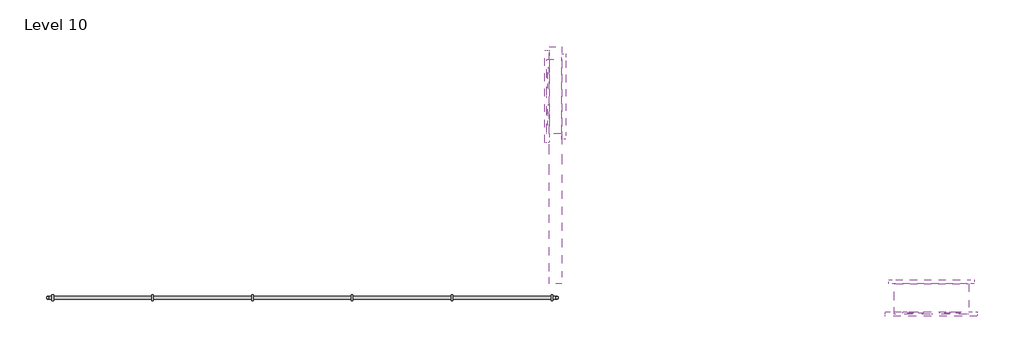
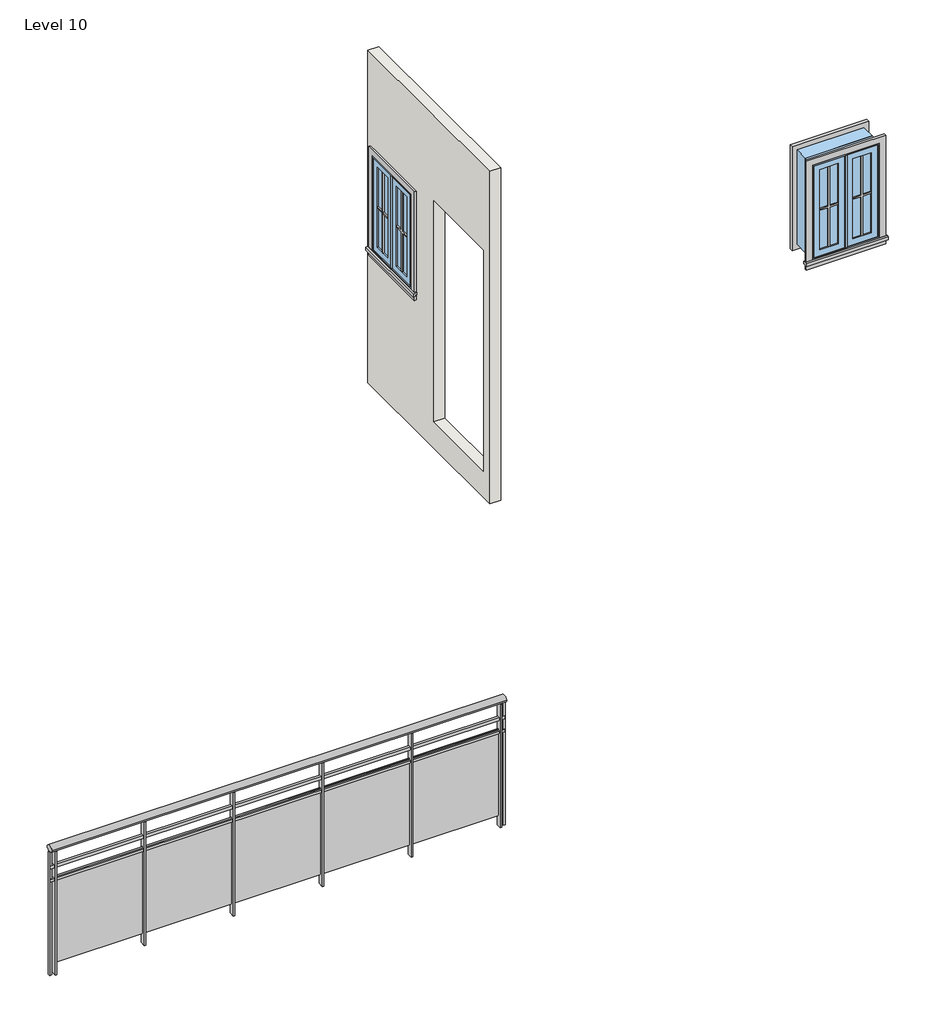
# One storey: 8 proxies, 2 windows, 1 railing, 1 wall.
"""IFC4 building model written with IfcOpenShell, lengths in millimetres."""

from ifc_helpers import new_model, si_unit, point, frame, origin, place, context, project, spatial, polyline, ellipse_curve, trimmed, outline, extrude, faceted_brep, transform, mapped, element, save
from ifc_brep_helpers import plane_surface, extruded_surface, advanced_brep
from components import muntin_pattern_2x2_muntin_pattern_2x2_53152e2c, muntin_pattern_2x2_muntin_pattern_2x2_e8f3e573, trim_window_exterior_flat_with_sill_a665a915, trim_window_interior_flat_picture_frame_d485c387, window_casement_double_3_c417fced, window_casement_double_3_e50e525e

model = new_model("IFC4")

# Units and contexts
model_context = context("Model", 3, world=origin())
ifc_project = project(units=[si_unit("LENGTHUNIT", "METRE", prefix="MILLI")], contexts=[model_context])

# Site, building, storey
site = spatial("IfcSite", under=ifc_project)
building = spatial("IfcBuilding", under=site)
storey = spatial("IfcBuildingStorey", under=building, Name="Level 10", Elevation=25603.2)

# Proxies
placement = place(None, origin())
muntin_pattern_2x2_muntin_pattern_2x2_shape = muntin_pattern_2x2_muntin_pattern_2x2_53152e2c(model_context)
element("IfcBuildingElementProxy", 1, Name="Muntin Pattern_2x2 : Muntin Pattern_2x2", ObjectType="Muntin Pattern_2x2 : Muntin Pattern_2x2", at=placement, inside=storey, context=model_context, shape_type="MappedRepresentation", body=[
    mapped(muntin_pattern_2x2_muntin_pattern_2x2_shape, transform((-1632.3904463, -4380.1669725, 30066.3460486), x_axis=(0.0, 1.0, 0.0), y_axis=(-1.0, 0.0, 0.0), z_axis=(0.0, 0.0, 1.0))),
])
element("IfcBuildingElementProxy", 2, Name="Muntin Pattern_2x2 : Muntin Pattern_2x2", ObjectType="Muntin Pattern_2x2 : Muntin Pattern_2x2", at=placement, inside=storey, context=model_context, shape_type="MappedRepresentation", body=[
    mapped(muntin_pattern_2x2_muntin_pattern_2x2_shape, transform((1620.3970537, -5972.4294725, 30245.05), x_axis=(-1.0, 0.0, 0.0), y_axis=(0.0, -1.0, 0.0), z_axis=(0.0, 0.0, 1.0))),
])
muntin_pattern_2x2_muntin_pattern_2x2_2_shape = muntin_pattern_2x2_muntin_pattern_2x2_e8f3e573(model_context)
element("IfcBuildingElementProxy", 3, Name="Muntin Pattern_2x2 : Muntin Pattern_2x2", ObjectType="Muntin Pattern_2x2 : Muntin Pattern_2x2", at=placement, inside=storey, context=model_context, shape_type="MappedRepresentation", body=[
    mapped(muntin_pattern_2x2_muntin_pattern_2x2_2_shape, transform((-1632.3904463, -4078.5419725, 30066.3460486), x_axis=(0.0, -1.0, 0.0), y_axis=(1.0, 0.0, 0.0), z_axis=(0.0, 0.0, 1.0))),
])
element("IfcBuildingElementProxy", 4, Name="Muntin Pattern_2x2 : Muntin Pattern_2x2", ObjectType="Muntin Pattern_2x2 : Muntin Pattern_2x2", at=placement, inside=storey, context=model_context, shape_type="MappedRepresentation", body=[
    mapped(muntin_pattern_2x2_muntin_pattern_2x2_2_shape, transform((1318.7720537, -5972.4294725, 30245.05), x_axis=(1.0, 0.0, 0.0), y_axis=(0.0, 1.0, 0.0), z_axis=(0.0, 0.0, 1.0))),
])
trim_window_exterior_flat_with_sill_shape = trim_window_exterior_flat_with_sill_a665a915(model_context)
element("IfcBuildingElementProxy", 5, Name="Trim-Window-Exterior-Flat : with Sill", ObjectType="Trim-Window-Exterior-Flat : with Sill", at=placement, inside=storey, context=model_context, shape_type="MappedRepresentation", body=[
    mapped(trim_window_exterior_flat_with_sill_shape, transform((-1641.9154463, -4229.3544725, 30910.8960486), x_axis=(0.0, -1.0, 0.0), y_axis=(0.0, 0.0, 1.0), z_axis=(-1.0, 0.0, 0.0))),
])
element("IfcBuildingElementProxy", 6, Name="Trim-Window-Exterior-Flat : with Sill", ObjectType="Trim-Window-Exterior-Flat : with Sill", at=placement, inside=storey, context=model_context, shape_type="MappedRepresentation", body=[
    mapped(trim_window_exterior_flat_with_sill_shape, transform((1469.5845537, -5981.9544725, 31089.6), x_axis=(1.0, 0.0, 0.0), y_axis=(0.0, 0.0, 1.0), z_axis=(0.0, -1.0, 0.0))),
])
trim_window_interior_flat_picture_frame_shape = trim_window_interior_flat_picture_frame_d485c387(model_context)
element("IfcBuildingElementProxy", 7, Name="Trim-Window-Interior-Flat : Picture Frame", ObjectType="Trim-Window-Interior-Flat : Picture Frame", at=placement, inside=storey, context=model_context, shape_type="MappedRepresentation", body=[
    mapped(trim_window_interior_flat_picture_frame_shape, transform((-1540.3154463, -4229.3544725, 30910.8960486), x_axis=(0.0, 1.0, 0.0), y_axis=(0.0, 0.0, 1.0), z_axis=(1.0, 0.0, 0.0))),
])
element("IfcBuildingElementProxy", 8, Name="Trim-Window-Interior-Flat : Picture Frame", ObjectType="Trim-Window-Interior-Flat : Picture Frame", at=placement, inside=storey, context=model_context, shape_type="MappedRepresentation", body=[
    mapped(trim_window_interior_flat_picture_frame_shape, transform((1469.5845537, -5753.3544725, 31089.6), x_axis=(-1.0, 0.0, 0.0), y_axis=(0.0, 0.0, 1.0), z_axis=(0.0, 1.0, 0.0))),
])

# Railing
element("IfcRailing", 9, ObjectType="Glass Panel - Bottom Fill", at=placement, inside=storey, context=model_context, shape_type="SolidModel", body=[
    advanced_brep(
    [(-5729.1673724, -5829.5544725, 26822.4), (-5729.1673724, -5905.7544725, 26822.4), (-1576.8982041, -5829.5544725, 26822.4), (-1576.8982041, -5905.7544725, 26822.4)],
    [
        (0, 1, ellipse_curve(frame((-5729.1673724, -5867.6544725, 26822.4), z_axis=(-1.0, 0.0, 0.0), x_axis=(0.0, -1.0, 0.0)), 38.1, 28.575)),
        (1, 0, ellipse_curve(frame((-5729.1673724, -5867.6544725, 26822.4), z_axis=(-1.0, 0.0, 0.0), x_axis=(0.0, -1.0, 0.0)), 38.1, 28.575)),
        (2, 3, ellipse_curve(frame((-1576.8982041, -5867.6544725, 26822.4), z_axis=(1.0, 0.0, 0.0), x_axis=(0.0, -1.0, 0.0)), 38.1, 28.575)),
        (3, 2, ellipse_curve(frame((-1576.8982041, -5867.6544725, 26822.4), z_axis=(1.0, 0.0, 0.0), x_axis=(0.0, -1.0, 0.0)), 38.1, 28.575)),
        (0, 2),
        (3, 1),
    ],
    [
        plane_surface(frame((-5729.1673724, -5867.6544725, 26822.4), z_axis=(-1.0, 0.0, 0.0), x_axis=(0.0, 1.0, 0.0))),
        plane_surface(frame((-1576.8982041, -5867.6544725, 26822.4), z_axis=(1.0, 0.0, 0.0), x_axis=(0.0, 1.0, 0.0))),
        extruded_surface(trimmed(ellipse_curve(frame((-1576.8982041, -5867.6544725, 26822.4), z_axis=(-1.0, 0.0, 0.0), x_axis=(0.0, -1.0, 0.0)), 38.1, 28.575), [point((-1576.8982041, -5829.5544725, 26822.4))], [point((-1576.8982041, -5905.7544725, 26822.4))], True, "CARTESIAN"), (-4152.2691683, 0.0, 0.0), 4152.2691683),
        extruded_surface(trimmed(ellipse_curve(frame((-1576.8982041, -5867.6544725, 26822.4), z_axis=(-1.0, 0.0, 0.0), x_axis=(0.0, -1.0, 0.0)), 38.1, 28.575), [point((-1576.8982041, -5905.7544725, 26822.4))], [point((-1576.8982041, -5829.5544725, 26822.4))], True, "CARTESIAN"), (-4152.2691683, 0.0, 0.0), 4152.2691683),
    ],
    [
        (0, [[1, 2]]),
        (1, [[3, 4]]),
        (2, [[-1, 5, -4, 6]]),
        (3, [[-2, -6, -3, -5]]),
    ],
),
    extrude(outline(polyline([(-5729.1673724, -5880.3544725), (-5729.1673724, -5854.9544725), (-1576.8982041, -5854.9544725), (-1576.8982041, -5880.3544725), (-5729.1673724, -5880.3544725)])), frame((0.0, 0.0, 26631.9), z_axis=(0.0, 0.0, 1.0), x_axis=(1.0, 0.0, 0.0)), (0.0, 0.0, 1.0), 25.4),
    extrude(outline(polyline([(-5729.1673724, -5880.3544725), (-5729.1673724, -5854.9544725), (-1576.8982041, -5854.9544725), (-1576.8982041, -5880.3544725), (-5729.1673724, -5880.3544725)])), frame((0.0, 0.0, 26504.9), z_axis=(0.0, 0.0, 1.0), x_axis=(1.0, 0.0, 0.0)), (0.0, 0.0, 1.0), 25.4),
    extrude(outline(polyline([(-1627.3827882, -5893.0544725), (-1627.3827882, -5842.2544725), (-1614.6827882, -5842.2544725), (-1614.6827882, -5893.0544725), (-1627.3827882, -5893.0544725)])), frame((0.0, 0.0, 25603.2), z_axis=(0.0, 0.0, 1.0), x_axis=(1.0, 0.0, 0.0)), (0.0, 0.0, 1.0), 1190.625),
    extrude(outline(polyline([(-2433.8327882, -5861.1193155), (-1621.0327882, -5861.1193155), (-1621.0327882, -5867.4693155), (-2433.8327882, -5867.4693155), (-2433.8327882, -5861.1193155)])), frame((0.0, 0.0, 25704.8), z_axis=(0.0, 0.0, 1.0), x_axis=(1.0, 0.0, 0.0)), (0.0, 0.0, 1.0), 838.2),
    extrude(outline(polyline([(-2440.1827882, -5893.0544725), (-2440.1827882, -5842.2544725), (-2427.4827882, -5842.2544725), (-2427.4827882, -5893.0544725), (-2440.1827882, -5893.0544725)])), frame((0.0, 0.0, 25603.2), z_axis=(0.0, 0.0, 1.0), x_axis=(1.0, 0.0, 0.0)), (0.0, 0.0, 1.0), 1190.625),
    extrude(outline(polyline([(-3246.6327882, -5861.1193155), (-2433.8327882, -5861.1193155), (-2433.8327882, -5867.4693155), (-3246.6327882, -5867.4693155), (-3246.6327882, -5861.1193155)])), frame((0.0, 0.0, 25704.8), z_axis=(0.0, 0.0, 1.0), x_axis=(1.0, 0.0, 0.0)), (0.0, 0.0, 1.0), 838.2),
    extrude(outline(polyline([(-3252.9827882, -5893.0544725), (-3252.9827882, -5842.2544725), (-3240.2827882, -5842.2544725), (-3240.2827882, -5893.0544725), (-3252.9827882, -5893.0544725)])), frame((0.0, 0.0, 25603.2), z_axis=(0.0, 0.0, 1.0), x_axis=(1.0, 0.0, 0.0)), (0.0, 0.0, 1.0), 1190.625),
    extrude(outline(polyline([(-4059.4327882, -5861.1193155), (-3246.6327882, -5861.1193155), (-3246.6327882, -5867.4693155), (-4059.4327882, -5867.4693155), (-4059.4327882, -5861.1193155)])), frame((0.0, 0.0, 25704.8), z_axis=(0.0, 0.0, 1.0), x_axis=(1.0, 0.0, 0.0)), (0.0, 0.0, 1.0), 838.2),
    extrude(outline(polyline([(-4065.7827882, -5893.0544725), (-4065.7827882, -5842.2544725), (-4053.0827882, -5842.2544725), (-4053.0827882, -5893.0544725), (-4065.7827882, -5893.0544725)])), frame((0.0, 0.0, 25603.2), z_axis=(0.0, 0.0, 1.0), x_axis=(1.0, 0.0, 0.0)), (0.0, 0.0, 1.0), 1190.625),
    extrude(outline(polyline([(-4872.2327882, -5861.1193155), (-4059.4327882, -5861.1193155), (-4059.4327882, -5867.4693155), (-4872.2327882, -5867.4693155), (-4872.2327882, -5861.1193155)])), frame((0.0, 0.0, 25704.8), z_axis=(0.0, 0.0, 1.0), x_axis=(1.0, 0.0, 0.0)), (0.0, 0.0, 1.0), 838.2),
    extrude(outline(polyline([(-4878.5827882, -5893.0544725), (-4878.5827882, -5842.2544725), (-4865.8827882, -5842.2544725), (-4865.8827882, -5893.0544725), (-4878.5827882, -5893.0544725)])), frame((0.0, 0.0, 25603.2), z_axis=(0.0, 0.0, 1.0), x_axis=(1.0, 0.0, 0.0)), (0.0, 0.0, 1.0), 1190.625),
    extrude(outline(polyline([(-5685.0327882, -5861.1193155), (-4872.2327882, -5861.1193155), (-4872.2327882, -5867.4693155), (-5685.0327882, -5867.4693155), (-5685.0327882, -5861.1193155)])), frame((0.0, 0.0, 25704.8), z_axis=(0.0, 0.0, 1.0), x_axis=(1.0, 0.0, 0.0)), (0.0, 0.0, 1.0), 838.2),
    extrude(outline(polyline([(-5691.3827882, -5893.0544725), (-5691.3827882, -5842.2544725), (-5678.6827882, -5842.2544725), (-5678.6827882, -5893.0544725), (-5691.3827882, -5893.0544725)])), frame((0.0, 0.0, 25603.2), z_axis=(0.0, 0.0, 1.0), x_axis=(1.0, 0.0, 0.0)), (0.0, 0.0, 1.0), 1190.625),
    extrude(outline(polyline([(-1589.5982041, -5877.1794725), (-1589.5982041, -5858.1294725), (-1570.5482041, -5858.1294725), (-1570.5482041, -5877.1794725), (-1589.5982041, -5877.1794725)])), frame((0.0, 0.0, 25603.2), z_axis=(0.0, 0.0, 1.0), x_axis=(1.0, 0.0, 0.0)), (0.0, 0.0, 1.0), 1190.625),
    extrude(outline(polyline([(-5735.5173724, -5877.1794725), (-5735.5173724, -5858.1294725), (-5716.4673724, -5858.1294725), (-5716.4673724, -5877.1794725), (-5735.5173724, -5877.1794725)])), frame((0.0, 0.0, 25603.2), z_axis=(0.0, 0.0, 1.0), x_axis=(1.0, 0.0, 0.0)), (0.0, 0.0, 1.0), 1190.625),
])

# Wall
element("IfcWall", 10, ObjectType="Generic - 4\"", at=placement, inside=storey, context=model_context, shape_type="Brep", body=[
    faceted_brep([(-1641.9154463, -3822.9544725, 28651.2), (-1641.9154463, -5753.3544725, 28651.2), (-1641.9154463, -5753.3544725, 28803.6), (-1641.9154463, -5753.3544725, 31851.6), (-1641.9154463, -5753.3544725, 31862.4896288), (-1641.9154463, -3822.9544725, 31862.4896288), (-1641.9154463, -5651.7544725, 28905.2), (-1641.9154463, -4864.3544725, 28905.2), (-1641.9154463, -4864.3544725, 31038.8), (-1641.9154463, -5651.7544725, 31038.8), (-1641.9154463, -3924.5544725, 30910.8960486), (-1641.9154463, -4534.1544725, 30910.8960486), (-1641.9154463, -4534.1544725, 29996.4960486), (-1641.9154463, -3924.5544725, 29996.4960486), (-1540.3154463, -3822.9544725, 28651.2), (-1540.3154463, -3822.9544725, 31862.4896288), (-1540.3154463, -5753.3544725, 31862.4896288), (-1540.3154463, -5753.3544725, 28651.2), (-1540.3154463, -5651.7544725, 28905.2), (-1540.3154463, -5651.7544725, 31038.8), (-1540.3154463, -4864.3544725, 31038.8), (-1540.3154463, -4864.3544725, 28905.2), (-1540.3154463, -3924.5544725, 30910.8960486), (-1540.3154463, -3924.5544725, 29996.4960486), (-1540.3154463, -4534.1544725, 29996.4960486), (-1540.3154463, -4534.1544725, 30910.8960486)], [[[0, 1, 2, 3, 4, 5], [6, 7, 8, 9], [10, 11, 12, 13]], [[14, 15, 16, 17], [18, 19, 20, 21], [22, 23, 24, 25]], [[1, 0, 14, 17]], [[5, 4, 16, 15]], [[0, 5, 15, 14]], [[4, 3, 2, 1, 17, 16]], [[7, 6, 18, 21]], [[8, 7, 21, 20]], [[9, 8, 20, 19]], [[6, 9, 19, 18]], [[23, 22, 10, 13]], [[24, 23, 13, 12]], [[25, 24, 12, 11]], [[22, 25, 11, 10]]]),
])

# Windows
window_casement_double_3_shape = window_casement_double_3_c417fced(model_context)
element("IfcWindow", 11, ObjectType="Window-Casement-Double : 3'", at=placement, inside=storey, context=model_context, shape_type="MappedRepresentation", body=[
    mapped(window_casement_double_3_shape, transform((1469.5845537, -5867.6544725, 29260.8), x_axis=(-1.0, 0.0, 0.0), y_axis=(0.0, -1.0, 0.0), z_axis=(0.0, 0.0, 1.0))),
])
window_casement_double_3_2_shape = window_casement_double_3_e50e525e(model_context)
element("IfcWindow", 12, ObjectType="Window-Casement-Double : 3'", at=placement, inside=storey, context=model_context, shape_type="MappedRepresentation", body=[
    mapped(window_casement_double_3_2_shape, transform((-1591.1154463, -4229.3544725, 29082.0960486), x_axis=(0.0, 1.0, 0.0), y_axis=(-1.0, 0.0, 0.0), z_axis=(0.0, 0.0, 1.0))),
])

save(model, "model.ifc")

# Revit data of these elements
# Type "Muntin Pattern_2x2 : Muntin Pattern_2x2"
#   Width [instance default] = 4' - 0"
#   Thickness = 0' - 0 1/2"
#   Height [instance default] = 4' - 0"
#   Distance = 0' - 0 3/4"
#   Interior Material [instance default] = none
#   Exterior Material [instance default] = none
#   Default Elevation = 0
# Type "Trim-Window-Exterior-Flat : with Sill"
#   Trim Width = 0' - 2 1/4"
#   Trim Thickness_Picture Frame = 0' - 1 1/4"
#   Trim Thickness_with Sill = 0' - 0 3/4"
#   Sill Thickness = 0' - 1 1/4"
#   Opening Width [instance default] = 2' - 0"
#   Opening Height [instance default] = 3' - 0"
#   Default Elevation = 4' - 0"
#   Sill = yes
#   Picture Frame = no
#   Trim Material [instance default] = none
# Type "Trim-Window-Interior-Flat : Picture Frame"
#   Trim Thickness_Picture Frame = 0' - 1 1/4"
#   Trim Width = 0' - 2 1/4"
#   Trim Thickness_with Sill = 0' - 0 3/4"
#   Sill Thickness = 0' - 1 1/4"
#   Opening Width [instance default] = 2' - 0"
#   Opening Height [instance default] = 3' - 0"
#   Default Elevation = 4' - 0"
#   Sill = no
#   Picture Frame = yes
#   Trim Material [instance default] = none
# Type "Glass Panel - Bottom Fill"
#   Assembly Code = "C2010400"
#   built-in parameter 1008612 = 0.0416667 (stored number, unit not read)
#   built-in parameter 1008611 = 0.0416667 (stored number, unit not read)
#   built-in parameter 1008609 = 0.333333 (stored number, unit not read)
#   built-in parameter 1008604 = 0.166667 (stored number, unit not read)
#   built-in parameter 1008603 = 0.166667 (stored number, unit not read)
#   Railing Height = 4' - 0"
#   built-in parameter 1008630 = 2
#   built-in parameter 1008610 = 2
#   built-in parameter 1008618 = Baluster - Square : 3/4"
# Type "Generic - 4\""
#   Assembly Code = "B2010"
#   Layers, outside or top first: 0' - 4" no material (function 1)
# Type "Window-Casement-Double : 3'"
#   Type Mark = "19"
#   Fire Rating = "0.5h"
#   Assembly Code = "B2020100"
#   Analytic Construction = "Double glazing - domestic"
#   Frame Extension [instance default] = 0' - 0 1/4"
#   Window Inset [instance default] = 0' - 0"
#   Wall Thickness [instance default] = 0' - 6"
#   Interior Wall Closure [instance default] = 0' - 2 1/4"
#   Half Width = 1' - 0"
#   Visual Light Transmittance = 0.81
#   Thermal Resistance (R) = 1.8146 (h·ft²·°F)/BTU
#   Solar Heat Gain Coefficient = 0.76
#   Rough Width = 2' - 0 1/2"
#   Rough Height = 3' - 0 1/2"
#   Height = 3' - 0"
#   Heat Transfer Coefficient (U) = 0.5511 BTU/(h·ft²·°F)
#   Exterior Wall Closure [instance default] = 0' - 1 1/4"
#   Extension Jamb [instance default] = 0' - 2 1/4"
#   Default Sill Height = 3' - 0"
#   Width = 2' - 0"
#   Muntin Visibility = yes
#   Interior Trim Visibility [instance default] = yes
#   Exterior Trim Visibility [instance default] = yes
#   Extension Jamb Visibility [instance default] = yes
#   Interior Trim Material = Wood - Stained
#   Muntin Pattern = Muntin Pattern_2x2 : Muntin Pattern_2x2
#   Interior Trim = Trim-Window-Interior-Flat : Picture Frame
#   Interior Frame Material = Wood - Stained
#   Glass Panel Material = Glass
#   Exterior Trim Material = Clad - White
#   Exterior Trim = Trim-Window-Exterior-Flat : with Sill
#   Exterior Frame Material = Clad - White
#   Wall Closure = (empty or 0)
# Elements 1, 2, 3, 4 (IfcBuildingElementProxy, "Muntin Pattern_2x2 : Muntin Pattern_2x2")
#   Width = 0' - 6 5/8"
#   Height = 2' - 6 1/2"
#   Interior Material = Wood - Stained
#   Exterior Material = Clad - White
#   Phase Created = New Construction
#   Materials on its faces: "Clad - White", "Wood - Stained"
# Elements 5, 6 (IfcBuildingElementProxy, "Trim-Window-Exterior-Flat : with Sill")
#   Opening Width = 2' - 0"
#   Opening Height = 3' - 0"
#   Trim Material = Clad - White
#   Phase Created = New Construction
#   Materials on its faces: "Clad - White"
# Elements 7, 8 (IfcBuildingElementProxy, "Trim-Window-Interior-Flat : Picture Frame")
#   Opening Width = 2' - 0"
#   Opening Height = 3' - 0"
#   Trim Material = Wood - Stained
#   Phase Created = New Construction
#   Materials on its faces: "Wood - Stained"
# Element 9 (IfcRailing, "Glass Panel - Bottom Fill")
#   Phase Created = New Construction
#   Materials on its faces: "Glass"
# Element 10 (IfcWall, "Generic - 4\"")
#   built-in parameter 1001111 = 10' - 0"
#   Top Offset = -0' - 5.57127"
#   Base Offset = 10' - 0"
#   wall height = 10' - 6.42873"
#   Phase Created = New Construction
#   Base Constraint = Level 10
#   Top Constraint = Level 31
#   Materials on its faces: "Default Wall"
# Element 11 (IfcWindow, "Window-Casement-Double : 3'")
#   Mark = "145"
#   Window Inset = 0' - 0"
#   Interior Wall Closure = 0' - 2 1/4"
#   Frame Extension = 0' - 0 1/4"
#   Exterior Wall Closure = 0' - 1 1/4"
#   Interior Trim Visibility = yes
#   Exterior Trim Visibility = yes
#   Phase Created = New Construction
#   Materials on its faces: "Wood - Stained", "Glass", "Clad - White"
# Element 12 (IfcWindow, "Window-Casement-Double : 3'")
#   Mark = "144"
#   Window Inset = 0' - 0"
#   Interior Wall Closure = 0' - 2 1/4"
#   Frame Extension = 0' - 0 1/4"
#   Exterior Wall Closure = 0' - 1 1/4"
#   Interior Trim Visibility = yes
#   Exterior Trim Visibility = yes
#   Phase Created = New Construction
#   Materials on its faces: "Wood - Stained", "Glass", "Clad - White"
# Materials
#   "Wood - Stained": class "Wood", colour RGB 224 178 126, transparency 0, Cost = 0
#   "Glass": class "Glass", colour RGB 0 128 192, transparency 0.75, Description = "Soda Lime Glass", Cost = 0
#   "Clad - White": class "Wood", colour RGB 242 242 238, transparency 0, Cost = 0
#   "Default Wall": colour RGB 128 128 128, transparency 0, Cost = 0
